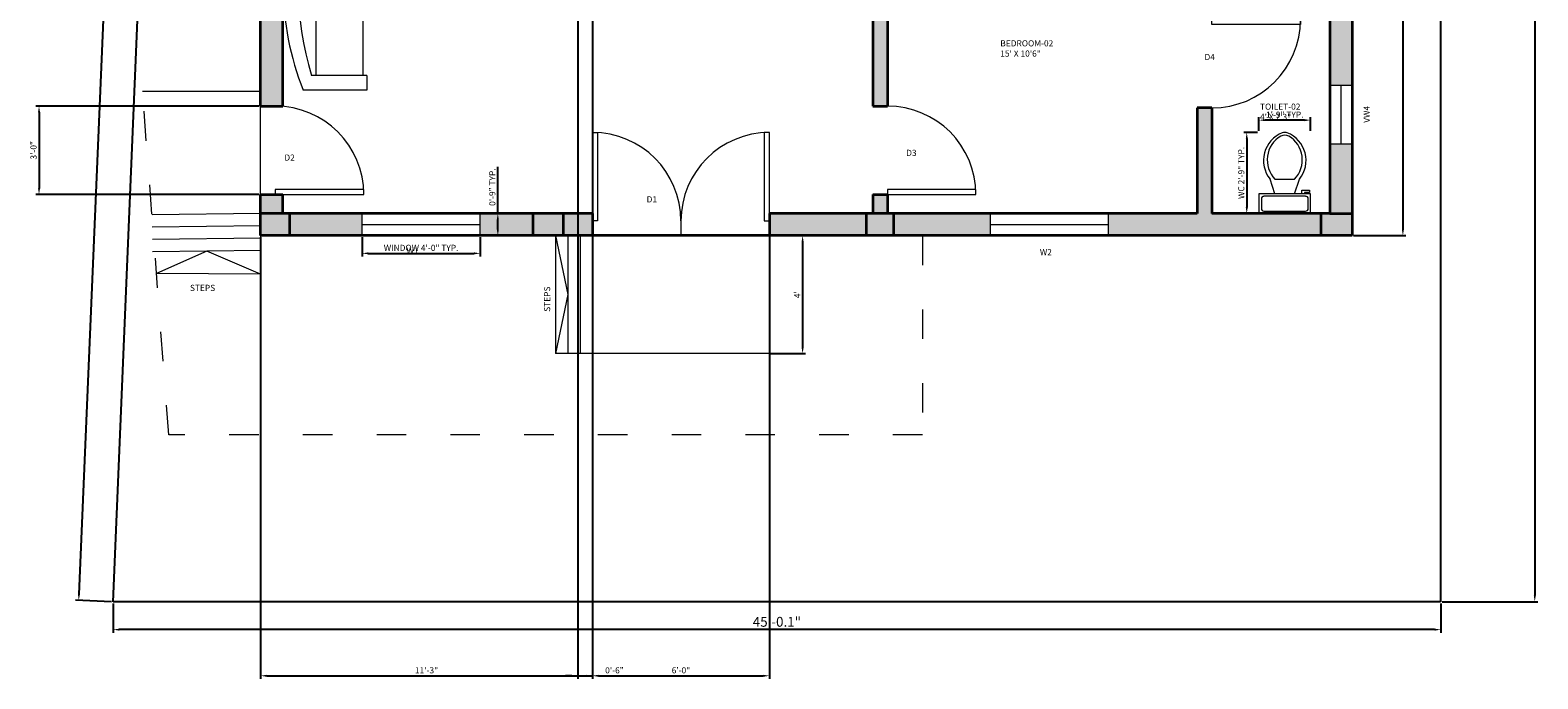
# Model space of a CAD drawing. Units: inches. Extents: x 5395 to 6469, y -203 to 448.
# Tile 1 of 7: x 5397 to 6010, y -186 to 78. Entities that reach past the tile are written whole.
import ezdxf

# ---------------------------------------------------------------- set-up
doc = ezdxf.new("R2010")
doc.units = ezdxf.units.IN
doc.linetypes.add('ACAD_ISO03W100', pattern=[30, 12, -18])
for name, color, linetype, lineweight in [('A-ANNO-DIMS', 2, 'Continuous', 18), ('A-ANNO-TEXT', 6, 'Continuous', 18), ('A-AREA-IDEN', 6, 'Continuous', 18), ('A-COLS', 7, 'Continuous', 35), ('A-COLS-PATT', 2, 'Continuous', 13), ('A-FLOR-FIXT', 70, 'Continuous', 18), ('A-FLOR-STRS', 3, 'Continuous', 18), ('A-GLAZ', 4, 'Continuous', 18), ('A-ROOF-OVHD', 1, 'ACAD_ISO03W100', 18), ('A-WALL', 7, 'Continuous', 35), ('A-WALL-PATT', 11, 'Continuous', 9), ('C-PROP', 7, 'Continuous', 25), ('door', 240, 'Continuous', 18), ('furniture', 70, 'Continuous', 18)]:
    doc.layers.add(name, color=color, linetype=linetype, lineweight=lineweight)
doc.styles.get("Standard").update_dxf_attribs({"font": 'arial.ttf'})
doc.dimstyles.new('ISO-25', dxfattribs={"dimtxt": 2.5, "dimasz": 2.5, "dimexe": 1.25, "dimexo": 0.625, "dimtad": 1, "dimdec": 1, "dimlunit": 3, "dimtxsty": 'Standard', "dimcen": 2.5, "dimadec": 0, "dimazin": 0, "dimtfac": 1, "dimtdec": 1, "dimtmove": 0, "dimatfit": 3, "dimfxl": 1, "dimarcsym": 0})

# ---------------------------------------------------------------- blocks, each defined once
blk = doc.blocks.new('*U2')
for p, q in [((0, 0), (0, -5)), ((30, 0), (30, -5))]:
    blk.add_line(p, q)
blk.add_lwpolyline([(0, 0), (0, 30), (1.75, 30), (1.75, 0)], close=True)
blk.add_arc((0, 0), 30, 0, 90)
blk = doc.blocks.new('*U3')
for p, q in [((-30, 0), (-30, -5)), ((0, 0), (0, -5))]:
    blk.add_line(p, q)
blk.add_lwpolyline([(0, 0), (0, 30), (-1.75, 30), (-1.75, 0)], close=True)
blk.add_arc((0, 0), 30, 90, 180)
blk = doc.blocks.new('*U5')
for p, q in [((-30, 0), (-30, 5)), ((0, 0), (0, 5))]:
    blk.add_line(p, q)
blk.add_lwpolyline([(0, 0), (0, -30), (-1.75, -30), (-1.75, 0)], close=True)
blk.add_arc((0, 0), 30, 180, 270)
blk = doc.blocks.new('*U4')
for p, q in [((0, 0), (0, 5)), ((30, 0), (30, 5))]:
    blk.add_line(p, q)
blk.add_lwpolyline([(0, 0), (0, -30), (1.75, -30), (1.75, 0)], close=True)
blk.add_arc((0, 0), 30, 270, 0)
blk = doc.blocks.new('Sofa - Roundback 7 ft.')
for p, q in [((-36.000027, -34), (-36.000027, -11.4696)), ((-12.00002, -32.4421), (-12.00003, -6.5971)), ((11.99997, -32.4421), (11.99998, -6.5971)), ((35.99998, -34), (35.99998, -11.4696)), ((-35.999844, -13.3819), (35.9998, -13.3819)), ((-36.000027, -32.4421), (35.99998, -32.4421))]:
    blk.add_line(p, q)
for points in [[(-36.000027, -34), (-42.000027, -34), (-42.000027, -8)], [(41.99998, -8), (41.99998, -34), (35.99998, -34)]]:
    blk.add_lwpolyline(points)
for centre, radius, start, end in [((0, -114.25), 114.25, 68.43141, 111.5686), ((-0.00001, -127.1968), 121.1968, 72.72033, 107.2797)]:
    blk.add_arc(centre, radius, start, end)
blk = doc.blocks.new('Toilet - top')
for p, q in [((9.5, -6), (9.5, -2)), ((-10, -8.5), (-8, -8.5)), ((-10, -9.5), (-10, -8.5)), ((-7, -9.5), (-10, -9.5)), ((-8, -8.5), (-8, -8)), ((-7, -8), (-7, -9.5)), ((-4, -8), (-6, -14)), ((4, -8), (6, -14)), ((4, -14), (-4, -14))]:
    blk.add_line(p, q)
blk.add_lwpolyline([(10.5, -8), (10.5, 0), (-10.5, 0), (-10.5, -8)], close=True)
for points in [[(-9.5, -2), (-9.5, -6)], [(8.5, -1), (-8.5, -1)], [(-8.5, -7), (8.5, -7)]]:
    blk.add_lwpolyline(points)
for centre, radius, start, end in [((-8.62, -1.88), 0.884, 81.8699, 188.1301), ((-8.62, -6.12), 0.884, 171.8699, 278.1301), ((8.62, -1.88), 0.884, 351.8699, 98.1301), ((8.62, -6.12), 0.884, 261.8699, 8.1301), ((3.52, -21.58), 12.17, 141.46911, 247.97143), ((4.2, -21.82), 11.33, 136.36773, 238.94682), ((-3.52, -21.58), 12.17, 292.02843, 38.53071), ((-4.2, -21.82), 11.33, 301.05301, 43.63209), ((0, -27.88), 4, 245.73182, 294.26817), ((0, -29), 4, 254.86053, 285.13947)]:
    blk.add_arc(centre, radius, start, end)
blk = doc.blocks.new('*D16')
at = {"layer": 'A-ANNO-DIMS', "color": 0, "lineweight": -2, "transparency": 16777216}
for p, q in [((5698.56, -5.69), (5712.67, -5.69)), ((5711.42, -8.19), (5711.42, -51.19)), ((5698.56, -53.69), (5712.67, -53.69))]:
    blk.add_line(p, q, dxfattribs=at)
at = {"layer": 'A-ANNO-DIMS', "color": 0, "transparency": 16777216}
for points in [[(5711.01, -8.19), (5711.84, -8.19), (5711.42, -5.69)], [(5711.01, -51.19), (5711.84, -51.19), (5711.42, -53.69)]]:
    blk.add_solid(points, dxfattribs=at)
at = {"layer": 'Defpoints', "color": 0, "transparency": 16777216}
for p in [(5697.94, -5.69), (5697.94, -53.69), (5711.42, -53.69)]:
    blk.add_point(p, dxfattribs=at)
at = {"layer": 'A-ANNO-DIMS', "color": 0, "transparency": 16777216, "insert": (5709.55, -29.69), "char_height": 2.5, "attachment_point": 5, "rotation": 90}
blk.add_mtext("4'", dxfattribs=at)
blk = doc.blocks.new('*D19')
at = {"layer": 'A-ANNO-DIMS', "color": 0, "lineweight": -2, "transparency": 16777216}
for p, q in [((5971.63, 414.31), (6010.49, 414.31)), ((6009.24, 411.81), (6009.24, -152.19)), ((5971.63, -154.69), (6010.49, -154.69))]:
    blk.add_line(p, q, dxfattribs=at)
at = {"layer": 'A-ANNO-DIMS', "color": 0, "transparency": 16777216}
for points in [[(6008.82, 411.81), (6009.65, 411.81), (6009.24, 414.31)], [(6008.82, -152.19), (6009.65, -152.19), (6009.24, -154.69)]]:
    blk.add_solid(points, dxfattribs=at)
at = {"layer": 'Defpoints', "color": 0, "transparency": 16777216}
for p in [(5971, 414.31), (5971, -154.69), (6009.24, -154.69)]:
    blk.add_point(p, dxfattribs=at)
at = {"layer": 'A-ANNO-DIMS', "color": 0, "transparency": 16777216, "insert": (6006.58, 129.81), "char_height": 4, "attachment_point": 5, "rotation": 90}
blk.add_mtext('47\'-5"', dxfattribs=at)
blk = doc.blocks.new('*D20')
at = {"layer": 'A-ANNO-DIMS', "color": 0, "lineweight": -2, "transparency": 16777216}
for p, q in [((5440.87, 412.4), (5417.08, -151.61)), ((5454.31, 414.33), (5439.73, 414.95)), ((5430.31, -154.67), (5415.73, -154.05))]:
    blk.add_line(p, q, dxfattribs=at)
at = {"layer": 'A-ANNO-DIMS', "color": 0, "transparency": 16777216}
for points in [[(5440.46, 412.41), (5441.29, 412.38), (5440.98, 414.89)], [(5416.67, -151.59), (5417.5, -151.63), (5416.98, -154.11)]]:
    blk.add_solid(points, dxfattribs=at)
at = {"layer": 'Defpoints', "color": 0, "transparency": 16777216}
for p in [(5454.94, 414.31), (5416.98, -154.11), (5430.94, -154.69)]:
    blk.add_point(p, dxfattribs=at)
at = {"layer": 'A-ANNO-DIMS', "color": 0, "transparency": 16777216, "insert": (5426.32, 130.51), "char_height": 4, "attachment_point": 5, "rotation": 87.58474}
blk.add_mtext('47\'-5.5"', dxfattribs=at)
blk = doc.blocks.new('*D21')
at = {"layer": 'A-ANNO-DIMS', "color": 0, "lineweight": -2, "transparency": 16777216}
for p, q in [((5430.94, -155.32), (5430.94, -167.27)), ((5971, -155.32), (5971, -167.27)), ((5968.5, -166.02), (5433.44, -166.02))]:
    blk.add_line(p, q, dxfattribs=at)
at = {"layer": 'A-ANNO-DIMS', "color": 0, "transparency": 16777216}
for points in [[(5433.44, -165.6), (5433.44, -166.43), (5430.94, -166.02)], [(5968.5, -165.6), (5968.5, -166.43), (5971, -166.02)]]:
    blk.add_solid(points, dxfattribs=at)
at = {"layer": 'Defpoints', "color": 0, "transparency": 16777216}
for p in [(5430.94, -154.69), (5971, -154.69), (5430.94, -166.02)]:
    blk.add_point(p, dxfattribs=at)
at = {"layer": 'A-ANNO-DIMS', "color": 0, "transparency": 16777216, "insert": (5700.97, -163.35), "char_height": 4, "attachment_point": 5}
blk.add_mtext('45\'-0.1"', dxfattribs=at)
blk = doc.blocks.new('*D22')
at = {"layer": 'A-ANNO-DIMS', "color": 0, "lineweight": -2, "transparency": 16777216}
for p, q in [((5935.56, 378.31), (5956.84, 378.31)), ((5955.59, 375.81), (5955.59, -3.19)), ((5935.56, -5.69), (5956.84, -5.69))]:
    blk.add_line(p, q, dxfattribs=at)
at = {"layer": 'A-ANNO-DIMS', "color": 0, "transparency": 16777216}
for points in [[(5955.17, 375.81), (5956, 375.81), (5955.59, 378.31)], [(5955.17, -3.19), (5956, -3.19), (5955.59, -5.69)]]:
    blk.add_solid(points, dxfattribs=at)
at = {"layer": 'Defpoints', "color": 0, "transparency": 16777216}
for p in [(5934.94, 378.31), (5934.94, -5.69), (5955.59, -5.69)]:
    blk.add_point(p, dxfattribs=at)
at = {"layer": 'A-ANNO-DIMS', "color": 0, "transparency": 16777216, "insert": (5952.92, 186.31), "char_height": 4, "attachment_point": 5, "rotation": 90}
blk.add_mtext("32'", dxfattribs=at)
blk = doc.blocks.new('WINDOW-48IN')
for p, q in [((0, 0), (0, 9)), ((48, 0), (48, 9)), ((0, 4.5), (48, 4.5))]:
    blk.add_line(p, q)
blk = doc.blocks.new('WINDOW-24IN')
for p, q in [((0, 24), (9, 24)), ((4.5, 0), (4.5, 24)), ((0, 0), (9, 0))]:
    blk.add_line(p, q)
blk = doc.blocks.new('*D31')
at = {"layer": 'A-ANNO-DIMS', "color": 0, "lineweight": -2, "transparency": 16777216}
for p, q in [((5532.25, -6.32), (5532.25, -14.14)), ((5580.25, -6.32), (5580.25, -14.14)), ((5534.75, -12.89), (5577.75, -12.89))]:
    blk.add_line(p, q, dxfattribs=at)
at = {"layer": 'A-ANNO-DIMS', "color": 0, "transparency": 16777216}
for points in [[(5534.75, -12.48), (5534.75, -13.31), (5532.25, -12.89)], [(5577.75, -12.48), (5577.75, -13.31), (5580.25, -12.89)]]:
    blk.add_solid(points, dxfattribs=at)
at = {"layer": 'Defpoints', "color": 0, "transparency": 16777216}
for p in [(5532.25, -5.69), (5580.25, -5.69), (5580.25, -12.89)]:
    blk.add_point(p, dxfattribs=at)
at = {"layer": 'A-ANNO-DIMS', "color": 0, "transparency": 16777216, "insert": (5556.25, -10.98), "char_height": 2.5, "attachment_point": 5}
blk.add_mtext('WINDOW 4\'-0" TYP.', dxfattribs=at)
blk = doc.blocks.new('*D32')
at = {"layer": 'A-ANNO-DIMS', "color": 0, "lineweight": -2, "transparency": 16777216}
for p, q in [((5587.45, 3.31), (5587.45, 22.29)), ((5580.88, 3.31), (5588.7, 3.31)), ((5587.45, -3.19), (5587.45, 0.81)), ((5580.88, -5.69), (5588.7, -5.69))]:
    blk.add_line(p, q, dxfattribs=at)
at = {"layer": 'A-ANNO-DIMS', "color": 0, "transparency": 16777216}
for points in [[(5587.04, 0.81), (5587.87, 0.81), (5587.45, 3.31)], [(5587.04, -3.19), (5587.87, -3.19), (5587.45, -5.69)]]:
    blk.add_solid(points, dxfattribs=at)
at = {"layer": 'Defpoints', "color": 0, "transparency": 16777216}
for p in [(5580.25, 3.31), (5587.45, 3.31), (5580.25, -5.69)]:
    blk.add_point(p, dxfattribs=at)
at = {"layer": 'A-ANNO-DIMS', "color": 0, "transparency": 16777216, "insert": (5585.55, 14.05), "char_height": 2.5, "attachment_point": 5, "rotation": 90}
blk.add_mtext('0\'-9" TYP.', dxfattribs=at)
blk = doc.blocks.new('*D49')
at = {"layer": 'A-ANNO-DIMS', "color": 0, "lineweight": -2, "transparency": 16777216}
for p, q in [((5896.42, 36.35), (5890.83, 36.35)), ((5892.08, 33.85), (5892.08, 5.81)), ((5896.42, 3.31), (5890.83, 3.31))]:
    blk.add_line(p, q, dxfattribs=at)
at = {"layer": 'A-ANNO-DIMS', "color": 0, "transparency": 16777216}
for points in [[(5891.67, 33.85), (5892.5, 33.85), (5892.08, 36.35)], [(5891.67, 5.81), (5892.5, 5.81), (5892.08, 3.31)]]:
    blk.add_solid(points, dxfattribs=at)
at = {"layer": 'Defpoints', "color": 0, "transparency": 16777216}
for p in [(5897.04, 36.35), (5892.08, 3.31), (5897.04, 3.31)]:
    blk.add_point(p, dxfattribs=at)
at = {"layer": 'A-ANNO-DIMS', "color": 0, "transparency": 16777216, "insert": (5890.17, 19.83), "char_height": 2.5, "attachment_point": 5, "rotation": 90}
blk.add_mtext('WC 2\'-9" TYP.', dxfattribs=at)
blk = doc.blocks.new('*D50')
at = {"layer": 'A-ANNO-DIMS', "color": 0, "lineweight": -2, "transparency": 16777216}
for p, q in [((5897.04, 36.98), (5897.04, 42.56)), ((5915.54, 41.31), (5899.54, 41.31)), ((5918.04, 36.98), (5918.04, 42.56))]:
    blk.add_line(p, q, dxfattribs=at)
at = {"layer": 'A-ANNO-DIMS', "color": 0, "transparency": 16777216}
for points in [[(5899.54, 41.72), (5899.54, 40.89), (5897.04, 41.31)], [(5915.54, 41.72), (5915.54, 40.89), (5918.04, 41.31)]]:
    blk.add_solid(points, dxfattribs=at)
at = {"layer": 'Defpoints', "color": 0, "transparency": 16777216}
for p in [(5897.04, 41.31), (5897.04, 36.35), (5918.04, 36.35)]:
    blk.add_point(p, dxfattribs=at)
at = {"layer": 'A-ANNO-DIMS', "color": 0, "transparency": 16777216, "insert": (5907.54, 43.21), "char_height": 2.5, "attachment_point": 5}
blk.add_mtext('1\'-9" TYP.', dxfattribs=at)
blk = doc.blocks.new('*D67')
at = {"layer": 'A-ANNO-DIMS', "color": 0, "lineweight": -2, "transparency": 16777216}
for p, q in [((5625.94, 2.68), (5625.94, -186.04)), ((5490.94, -6.32), (5490.94, -186.04)), ((5493.44, -184.79), (5623.44, -184.79))]:
    blk.add_line(p, q, dxfattribs=at)
at = {"layer": 'A-ANNO-DIMS', "color": 0, "transparency": 16777216}
for points in [[(5493.44, -184.38), (5493.44, -185.21), (5490.94, -184.79)], [(5623.44, -184.38), (5623.44, -185.21), (5625.94, -184.79)]]:
    blk.add_solid(points, dxfattribs=at)
at = {"layer": 'Defpoints', "color": 0, "transparency": 16777216}
for p in [(5625.94, 3.31), (5490.94, -5.69), (5625.94, -184.79)]:
    blk.add_point(p, dxfattribs=at)
at = {"layer": 'A-ANNO-DIMS', "color": 0, "transparency": 16777216, "insert": (5558.44, -182.89), "char_height": 2.5, "attachment_point": 5}
blk.add_mtext('11\'-3"', dxfattribs=at)
blk = doc.blocks.new('*D68')
at = {"layer": 'A-ANNO-DIMS', "color": 0, "lineweight": -2, "transparency": 16777216}
for p, q in [((5625.94, 2.68), (5625.94, -186.04)), ((5697.94, 2.68), (5697.94, -186.04)), ((5628.44, -184.79), (5695.44, -184.79))]:
    blk.add_line(p, q, dxfattribs=at)
at = {"layer": 'A-ANNO-DIMS', "color": 0, "transparency": 16777216}
for points in [[(5628.44, -184.38), (5628.44, -185.21), (5625.94, -184.79)], [(5695.44, -184.38), (5695.44, -185.21), (5697.94, -184.79)]]:
    blk.add_solid(points, dxfattribs=at)
at = {"layer": 'Defpoints', "color": 0, "transparency": 16777216}
for p in [(5625.94, 3.31), (5697.94, 3.31), (5697.94, -184.79)]:
    blk.add_point(p, dxfattribs=at)
at = {"layer": 'A-ANNO-DIMS', "color": 0, "transparency": 16777216, "insert": (5661.94, -182.89), "char_height": 2.5, "attachment_point": 5}
blk.add_mtext('6\'-0"', dxfattribs=at)
blk = doc.blocks.new('*D69')
at = {"layer": 'A-ANNO-DIMS', "color": 0, "lineweight": -2, "transparency": 16777216}
for p, q in [((5490.31, 47.04), (5399.59, 47.04)), ((5400.84, 44.54), (5400.84, 13.54)), ((5490.31, 11.04), (5399.59, 11.04))]:
    blk.add_line(p, q, dxfattribs=at)
at = {"layer": 'A-ANNO-DIMS', "color": 0, "transparency": 16777216}
for points in [[(5400.42, 44.54), (5401.25, 44.54), (5400.84, 47.04)], [(5400.42, 13.54), (5401.25, 13.54), (5400.84, 11.04)]]:
    blk.add_solid(points, dxfattribs=at)
at = {"layer": 'Defpoints', "color": 0, "transparency": 16777216}
for p in [(5490.94, 47.04), (5400.84, 11.04), (5490.94, 11.04)]:
    blk.add_point(p, dxfattribs=at)
at = {"layer": 'A-ANNO-DIMS', "color": 0, "transparency": 16777216, "insert": (5398.93, 29.04), "char_height": 2.5, "attachment_point": 5, "rotation": 90}
blk.add_mtext('3\'-0"', dxfattribs=at)
blk = doc.blocks.new('*D72')
at = {"layer": 'A-ANNO-DIMS', "color": 0, "lineweight": -2, "transparency": 16777216}
for p, q in [((5619.94, 236.68), (5619.94, -186.04)), ((5625.94, 236.68), (5625.94, -186.04)), ((5617.44, -184.79), (5614.94, -184.79)), ((5619.94, -184.79), (5625.94, -184.79)), ((5628.44, -184.79), (5638.83, -184.79))]:
    blk.add_line(p, q, dxfattribs=at)
at = {"layer": 'A-ANNO-DIMS', "color": 0, "transparency": 16777216}
for points in [[(5617.44, -184.38), (5617.44, -185.21), (5619.94, -184.79)], [(5628.44, -184.38), (5628.44, -185.21), (5625.94, -184.79)]]:
    blk.add_solid(points, dxfattribs=at)
at = {"layer": 'Defpoints', "color": 0, "transparency": 16777216}
for p in [(5619.94, 237.31), (5625.94, 237.31), (5625.94, -184.79)]:
    blk.add_point(p, dxfattribs=at)
at = {"layer": 'A-ANNO-DIMS', "color": 0, "transparency": 16777216, "insert": (5634.88, -182.89), "char_height": 2.5, "attachment_point": 5}
blk.add_mtext('0\'-6"', dxfattribs=at)

msp = doc.modelspace()

# ---------------------------------------------------------------- hatches: boundary and pattern name
at = {"layer": 'A-COLS-PATT'}
h = msp.add_hatch(color=256, dxfattribs=at)
h.dxf.hatch_style = 1
h.paths.add_polyline_path([(5502.78, 3.31), (5499.94, 3.31), (5490.94, 3.31), (5490.94, -5.69), (5502.78, -5.69)])
h = msp.add_hatch(color=256, dxfattribs=at)
h.dxf.hatch_style = 1
h.paths.add_polyline_path([(5614.13, 3.31), (5601.84, 3.31), (5601.84, -5.69), (5614.13, -5.69)])
h = msp.add_hatch(color=256, dxfattribs=at)
h.dxf.hatch_style = 1
h.paths.add_polyline_path([(5748.46, 3.31), (5737.31, 3.31), (5737.31, -5.69), (5748.46, -5.69)])
h = msp.add_hatch(color=256, dxfattribs=at)
h.dxf.hatch_style = 1
h.paths.add_polyline_path([(5934.94, 3.31), (5925.94, 3.31), (5922.21, 3.31), (5922.21, -5.69), (5934.94, -5.69)])
at = {"layer": 'A-WALL-PATT'}
h = msp.add_hatch(color=256, dxfattribs=at)
h.dxf.hatch_style = 1
h.paths.add_polyline_path([(5538.88, 378.31), (5499.94, 378.31), (5499.94, 369.31), (5538.88, 369.31)])
h.paths.add_polyline_path([(5499.94, 276.14), (5490.94, 276.14), (5490.94, 227.71), (5499.94, 227.71), (5499.94, 237.31)])
h.paths.add_polyline_path([(5565.94, 243.31), (5499.94, 243.31), (5499.94, 237.31), (5559.94, 237.31), (5559.94, 225.31), (5565.94, 225.31)])
h.paths.add_polyline_path([(5625.94, 367.55), (5619.94, 367.55), (5619.94, 237.31), (5625.94, 237.31)])
h.paths.add_polyline_path([(5745.94, 369.31), (5739.94, 369.31), (5739.94, 237.31), (5745.94, 237.31)])
h.paths.add_polyline_path([(5745.94, 192.25), (5739.94, 192.25), (5739.94, 190.23), (5745.94, 190.23)])
h.paths.add_polyline_path([(5745.94, 180.33), (5739.94, 180.33), (5739.94, 47.04), (5745.94, 47.04)])
h.paths.add_polyline_path([(5877.94, 183.31), (5884.03, 183.31), (5884.03, 189.31), (5747.34, 189.31), (5747.34, 183.31), (5871.94, 183.31), (5871.94, 82.27), (5877.94, 82.27), (5877.94, 90.31), (5925.94, 90.31), (5925.94, 96.31), (5877.94, 96.31)])
h.paths.add_polyline_path([(5934.94, 128.85), (5925.94, 128.85), (5925.94, 55.61), (5934.94, 55.61)])
h.paths.add_polyline_path([(5934.94, 181.4), (5925.94, 181.4), (5925.94, 152.85), (5934.94, 152.85)])
h.paths.add_polyline_path([(5925.94, 189.31), (5914.03, 189.31), (5914.03, 183.31), (5925.94, 183.31)], flags=17)
h.paths.add_polyline_path([(5934.94, 369.31), (5925.94, 369.31), (5925.94, 237.31), (5934.94, 237.31)])
h.paths.add_polyline_path([(5657.93, 378.31), (5627.19, 378.31), (5627.19, 369.31), (5657.93, 369.31)])
h.paths.add_polyline_path([(5619.94, 378.31), (5586.88, 378.31), (5586.88, 369.31), (5619.94, 369.31)])
h.paths.add_polyline_path([(5739.94, 378.31), (5705.93, 378.31), (5705.93, 369.31), (5739.94, 369.31)])
h.paths.add_polyline_path([(5812.1, 378.31), (5753.55, 378.31), (5753.55, 369.31), (5812.1, 369.31)])
h.paths.add_polyline_path([(5923.7, 378.31), (5860.1, 378.31), (5860.1, 369.31), (5923.7, 369.31)])
h.paths.add_polyline_path([(5499.94, 203.71), (5490.94, 203.71), (5490.94, 189.31), (5499.94, 189.31)])
h.paths.add_polyline_path([(5612.93, 189.31), (5499.94, 189.31), (5499.94, 183.31), (5612.93, 183.31)])
h.paths.add_polyline_path([(5499.94, 178.42), (5490.94, 178.42), (5490.94, 132.59), (5499.94, 132.59)])
h.paths.add_polyline_path([(5499.94, 84.59), (5490.94, 84.59), (5490.94, 47.04), (5499.94, 47.04)])
h.paths.add_polyline_path([(5499.94, 11.04), (5490.94, 11.04), (5490.94, 3.31), (5499.94, 3.31)])
h.paths.add_polyline_path([(5532.25, 3.31), (5502.78, 3.31), (5502.78, -5.69), (5532.25, -5.69)])
h.paths.add_polyline_path([(5601.84, 3.31), (5580.25, 3.31), (5580.25, -5.69), (5601.84, -5.69)])
h.paths.add_polyline_path([(5625.94, 3.31), (5614.13, 3.31), (5614.13, -5.69), (5625.94, -5.69)])
h.paths.add_polyline_path([(5787.9, 3.31), (5748.46, 3.31), (5748.46, -5.69), (5787.9, -5.69)])
h.paths.add_polyline_path([(5737.31, 3.31), (5697.94, 3.31), (5697.94, -5.69), (5737.31, -5.69)])
h.paths.add_polyline_path([(5745.94, 11.04), (5739.94, 11.04), (5739.94, 3.31), (5745.94, 3.31)])
h.paths.add_polyline_path([(5922.21, 3.31), (5877.94, 3.31), (5877.94, 46.27), (5871.94, 46.27), (5871.94, 3.31), (5835.9, 3.31), (5835.9, -5.69), (5922.21, -5.69)])
h.paths.add_polyline_path([(5934.94, 31.61), (5925.94, 31.61), (5925.94, 3.31), (5934.94, 3.31)])

# ---------------------------------------------------------------- linework, layer by layer
at = {"layer": 'A-COLS'}
for p, q in [((5499.94, 3.31), (5490.94, 3.31)), ((5502.78, 3.31), (5502.78, -5.69)), ((5601.84, -5.69), (5601.84, 3.31)), ((5614.13, -5.69), (5614.13, 3.31)), ((5737.31, 3.31), (5737.31, -5.69)), ((5748.46, 3.31), (5748.46, -5.69)), ((5922.21, 3.31), (5922.21, -5.69)), ((5925.94, 3.31), (5934.94, 3.31))]:
    msp.add_line(p, q, dxfattribs=at)
at = {"layer": 'A-FLOR-STRS'}
for p, q in [((5490.94, 53.03), (5442.94, 53.03)), ((5490.94, 3.31), (5446.8, 2.72)), ((5490.94, 3.31), (5490.94, -21.35)), ((5491, -1.69), (5446.86, -2.28)), ((5610.94, -5.69), (5610.94, -53.69)), ((5610.94, -5.69), (5615.94, -29.69)), ((5615.94, -5.69), (5615.94, -53.69)), ((5620.94, -5.69), (5620.94, -53.69)), ((5625.94, -5.69), (5625.94, -53.69)), ((5697.94, -5.69), (5697.94, -53.69)), ((5491.07, -6.69), (5446.93, -7.28)), ((5491.13, -11.69), (5446.99, -12.28)), ((5469.06, -11.98), (5448.63, -21.14)), ((5490.94, -21.35), (5469.06, -11.98)), ((5490.94, -21.35), (5448.63, -21.14)), ((5615.94, -29.69), (5610.94, -53.69)), ((5697.94, -53.69), (5610.94, -53.69))]:
    msp.add_line(p, q, dxfattribs=at)
at = {"layer": 'A-ROOF-OVHD'}
for p, q in [((5453.66, -86.69), (5442.94, 53.03)), ((5760.19, -5.69), (5760.19, -86.69)), ((5760.19, -86.69), (5453.66, -86.69))]:
    msp.add_line(p, q, dxfattribs=at)
at = {"layer": 'A-WALL'}
for p, q in [((5490.94, 47.04), (5490.94, 378.31)), ((5934.94, 378.31), (5934.94, -5.69)), ((5499.94, 47.04), (5499.94, 369.31)), ((5925.94, 369.31), (5925.94, 3.31)), ((5739.94, 192.25), (5739.94, 47.04)), ((5745.94, 183.31), (5745.94, 47.04)), ((5490.94, 47.04), (5499.94, 47.04)), ((5739.94, 47.04), (5745.94, 47.04)), ((5877.94, 46.27), (5871.94, 46.27)), ((5871.94, 46.27), (5871.94, 3.31)), ((5877.94, 46.27), (5877.94, 3.31)), ((5490.94, -5.69), (5490.94, 11.04)), ((5490.94, 11.04), (5499.94, 11.04)), ((5499.94, 3.31), (5499.94, 11.04)), ((5739.94, 11.04), (5745.94, 11.04)), ((5739.94, 11.04), (5739.94, 3.31)), ((5745.94, 11.04), (5745.94, 3.31)), ((5625.94, 3.31), (5499.94, 3.31)), ((5625.94, 3.31), (5625.94, -5.69)), ((5871.94, 3.31), (5697.94, 3.31)), ((5697.94, 3.31), (5697.94, -5.69)), ((5925.94, 3.31), (5877.94, 3.31)), ((5934.94, -5.69), (5490.94, -5.69))]:
    msp.add_line(p, q, dxfattribs=at)
at = {"layer": 'C-PROP'}
for p, q in [((5430.94, -154.69), (5454.94, 414.31)), ((5970.94, 414.31), (5970.94, -154.69)), ((5970.94, -154.69), (5430.94, -154.69)), ((5970.94, -154.69), (5430.94, -154.69))]:
    msp.add_line(p, q, dxfattribs=at)
at = {"layer": 'door'}
for p, q in [((5490.94, 11.04), (5490.94, 47.04)), ((5625.94, -5.69), (5661.94, -5.69))]:
    msp.add_line(p, q, dxfattribs=at)

# ---------------------------------------------------------------- block references
at = {"layer": 'A-FLOR-FIXT', "rotation": 180}
msp.add_blockref('Toilet - top', (5907.54, 3.31), dxfattribs=at)
at = {"layer": 'A-GLAZ'}
for name, p in [('WINDOW-24IN', (5925.94, 31.61)), ('WINDOW-48IN', (5532.25, -5.69)), ('WINDOW-48IN', (5787.9, -5.69))]:
    msp.add_blockref(name, p, dxfattribs=at)
at = {"layer": 'door', "rotation": 90}
for name, p, xscale, yscale, zscale in [('*U5', (5877.94, 82.27), 1.199999999999999, 1.199999999999999, 1.199999999999999), ('*U4', (5496.94, 11.04), 1.200014089153335, 1.200014089153335, 1.200014089153335), ('*U4', (5745.94, 11.04), 1.2, 1.2, 1.2)]:
    msp.add_blockref(name, p, dxfattribs=dict(at, xscale=xscale, yscale=yscale, zscale=zscale))
at = {"layer": 'door', "xscale": 1.199999999999999, "yscale": 1.199999999999999, "zscale": 1.199999999999999}
for name, p in [('*U2', (5625.94, 0.31)), ('*U3', (5697.94, 0.31))]:
    msp.add_blockref(name, p, dxfattribs=at)
at = {"layer": 'furniture', "rotation": 90}
msp.add_blockref('Sofa - Roundback 7 ft.', (5500.23, 95.49), dxfattribs=at)

# ---------------------------------------------------------------- texts
at = {"layer": 'A-ANNO-TEXT', "char_height": 2.5, "attachment_point": 1}
for s, insert in [('D4', (5874.89, 68.27)), ('D2', (5500.63, 27.33)), ('D3', (5753.56, 29.25)), ('D1', (5647.98, 10.33)), ('W1', (5550.32, -10.53)), ('W2', (5807.94, -11.16)), ('STEPS', (5462.22, -25.69))]:
    msp.add_mtext_dynamic_manual_height_columns(s, width=62.1492, gutter_width=12.5, heights=[0], dxfattribs=dict(at, insert=insert))
at = {"layer": 'A-ANNO-TEXT', "char_height": 2.5, "attachment_point": 1, "rotation": 90}
for s, insert in [('VW4', (5939.61, 40.25)), ('STEPS', (5606.25, -36.67))]:
    msp.add_mtext_dynamic_manual_height_columns(s, width=62.1492, gutter_width=12.5, heights=[0], dxfattribs=dict(at, insert=insert))
at = {"layer": 'A-AREA-IDEN', "char_height": 2.5, "attachment_point": 1}
for s, insert in [('BEDROOM-02\\P15\' X 10\'6"', (5791.83, 73.82)), ('TOILET-02\\P4\' X 7\'3"', (5897.47, 48.05))]:
    msp.add_mtext_dynamic_manual_height_columns(s, width=62.1492, gutter_width=12.5, heights=[0], dxfattribs=dict(at, insert=insert))

# ---------------------------------------------------------------- dimensions: what is measured, and where the dimension line sits
at = {"layer": 'A-ANNO-DIMS'}
for p1, p2, distance, picture, middle in [((5454.94, 414.31), (5430.94, -154.69), -13.97, '*D20', (5426.32, 130.51)), ((5971, 414.31), (5971, -154.69), 38.23, '*D19', (6006.58, 129.81))]:
    dim = msp.add_aligned_dim(p1=p1, p2=p2, distance=distance, dimstyle='ISO-25', override={"dimtxt": 4, "dimclrd": 0, "dimclre": 0, "dimclrt": 0}, dxfattribs=at)
    dim.commit()
    dim.dimension.update_dxf_attribs({"geometry": picture, "text_midpoint": middle})
for base, p1, p2, override, picture, middle in [((5955.59, -5.69), (5934.94, 378.31), (5934.94, -5.69), {"dimtxt": 4, "dimclrd": 0, "dimclre": 0, "dimclrt": 0}, '*D22', (5952.92, 186.31)), ((5400.84, 11.04), (5490.94, 47.04), (5490.94, 11.04), {"dimdec": 1, "dimlfac": 1, "dimrnd": 0, "dimzin": 1, "dimdsep": 46, "dimlunit": 4, "dimfrac": 2}, '*D69', (5398.93, 29.04)), ((5711.42, -53.69), (5697.94, -5.69), (5697.94, -53.69), {"dimclrd": 0, "dimclre": 0, "dimclrt": 0}, '*D16', (5709.55, -29.69))]:
    dim = msp.add_linear_dim(base=base, p1=p1, p2=p2, angle=90, dimstyle='ISO-25', override=override, dxfattribs=at)
    dim.commit()
    dim.dimension.update_dxf_attribs({"geometry": picture, "text_midpoint": middle})
for base, p1, p2, override, picture, middle in [((5625.94, -184.79), (5619.94, 237.31), (5625.94, 237.31), {"dimdec": 1, "dimlfac": 1, "dimrnd": 0, "dimzin": 1, "dimdsep": 46, "dimlunit": 4, "dimfrac": 2}, '*D72', (5634.88, -182.89)), ((5625.94, -184.79), (5490.94, -5.69), (5625.94, 3.31), {"dimdec": 1, "dimlfac": 1, "dimrnd": 0, "dimzin": 1, "dimdsep": 46, "dimlunit": 4, "dimfrac": 2}, '*D67', (5558.44, -182.89)), ((5697.94, -184.79), (5625.94, 3.31), (5697.94, 3.31), {"dimdec": 1, "dimlfac": 1, "dimrnd": 0, "dimzin": 1, "dimdsep": 46, "dimlunit": 4, "dimfrac": 2}, '*D68', (5661.94, -182.89)), ((5430.94, -166.02), (5971, -154.69), (5430.94, -154.69), {"dimtxt": 4, "dimclrd": 0, "dimclre": 0, "dimclrt": 0}, '*D21', (5700.97, -163.35))]:
    dim = msp.add_linear_dim(base=base, p1=p1, p2=p2, dimstyle='ISO-25', override=override, dxfattribs=at)
    dim.commit()
    dim.dimension.update_dxf_attribs({"geometry": picture, "text_midpoint": middle})
for base, p1, p2, angle, text, picture, middle in [((5897.04, 41.31), (5918.04, 36.35), (5897.04, 36.35), 180, '<> TYP.', '*D50', (5907.54, 43.21)), ((5892.08, 3.31), (5897.04, 36.35), (5897.04, 3.31), 270, 'WC <> TYP.', '*D49', (5890.17, 19.83)), ((5587.45, 3.31), (5580.25, -5.69), (5580.25, 3.31), 90, '<> TYP.', '*D32', (5585.55, 14.05))]:
    dim = msp.add_linear_dim(base=base, p1=p1, p2=p2, angle=angle, text=text, dimstyle='ISO-25', override={"dimdec": 1, "dimlfac": 1, "dimrnd": 0, "dimzin": 1, "dimdsep": 46, "dimlunit": 4, "dimfrac": 2}, dxfattribs=at)
    dim.commit()
    dim.dimension.update_dxf_attribs({"geometry": picture, "text_midpoint": middle})
dim = msp.add_linear_dim(base=(5580.25, -12.89), p1=(5532.25, -5.69), p2=(5580.25, -5.69), text='WINDOW <> TYP.', dimstyle='ISO-25', override={"dimdec": 1, "dimlfac": 1, "dimrnd": 0, "dimzin": 1, "dimdsep": 46, "dimlunit": 4, "dimfrac": 2}, dxfattribs=at)
dim.commit()
dim.dimension.update_dxf_attribs({"geometry": '*D31', "text_midpoint": (5556.25, -10.98)})

doc.saveas('drawing.dxf')
